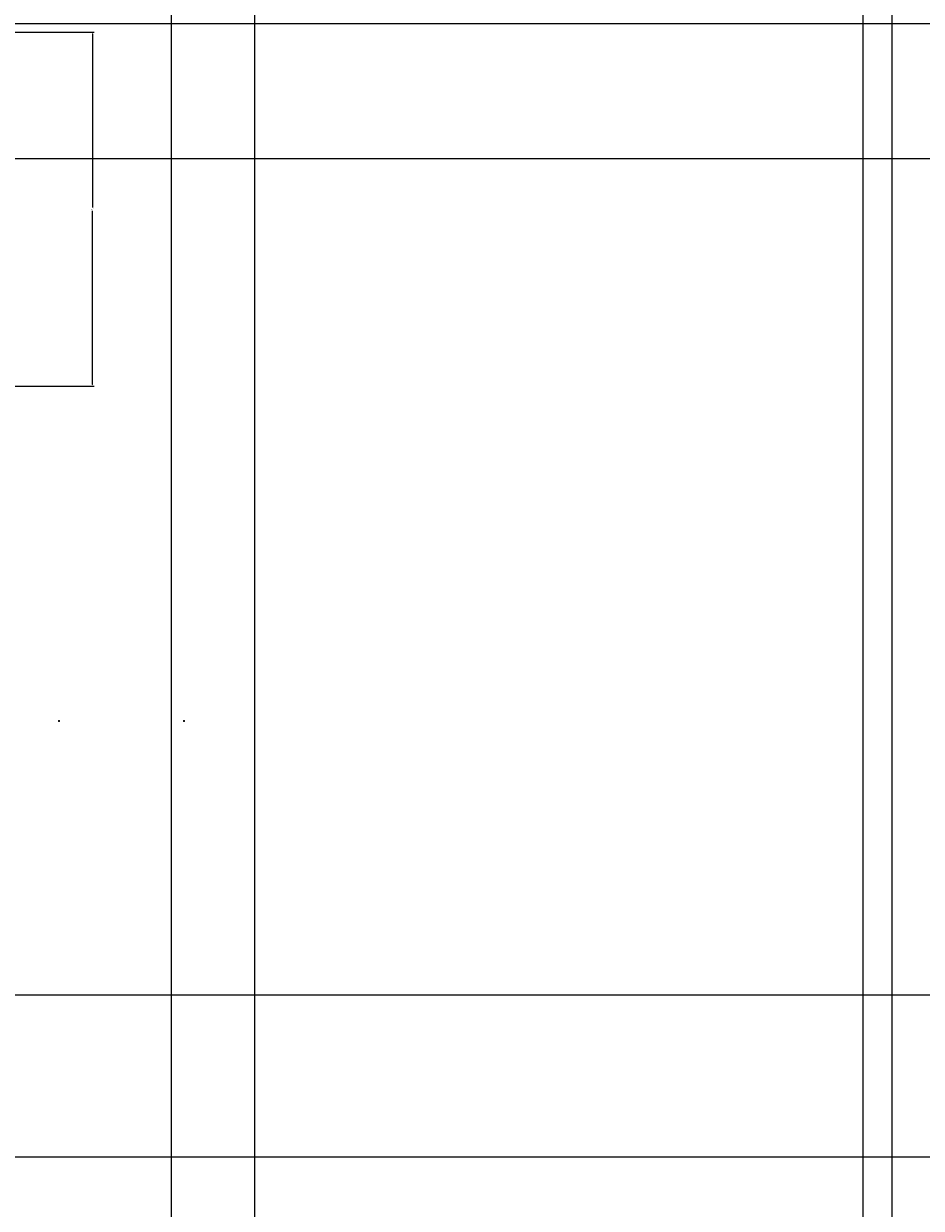
# Model space of a CAD drawing. Units: inches. Extents: x 1201 to 1754, y 247 to 775.
# Tile 5 of 10: x 1382 to 1475, y 435 to 557. Entities that reach past the tile are written whole.
import ezdxf

# ---------------------------------------------------------------- set-up
doc = ezdxf.new("R2010")
doc.units = ezdxf.units.IN
doc.layers.add('A-ANNO-DIMS', color=2, linetype='Continuous', lineweight=18)
doc.styles.get("Standard").update_dxf_attribs({"font": 'arial.ttf'})
doc.dimstyles.get("Standard").update_dxf_attribs({"dimtxt": 0.18, "dimasz": 0.18, "dimexe": 0.18, "dimexo": 0.0625, "dimgap": 0.09, "dimtad": 0, "dimtih": 1, "dimtoh": 1, "dimdec": 4, "dimzin": 0, "dimdsep": 46, "dimtxsty": 'Standard', "dimcen": 0.09, "dimadec": 0, "dimazin": 0, "dimtfac": 1, "dimtdec": 4, "dimtofl": 0, "dimtmove": 0, "dimatfit": 3, "dimfxl": 1, "dimtolj": 1, "dimtzin": 0, "dimarcsym": 0})

# ---------------------------------------------------------------- blocks, each defined once
blk = doc.blocks.new('*D32')
at = {"layer": 'A-ANNO-DIMS', "color": 0, "lineweight": -2, "transparency": 16777216}
for p, q in [((1379.77, 556.57), (1388.89, 556.57)), ((1388.71, 556.39), (1388.71, 538.42)), ((1388.71, 520.08), (1388.71, 538.05)), ((1379.77, 519.9), (1388.89, 519.9))]:
    blk.add_line(p, q, dxfattribs=at)
at = {"layer": 'A-ANNO-DIMS', "color": 0, "transparency": 16777216}
for points in [[(1388.68, 556.39), (1388.74, 556.39), (1388.71, 556.57)], [(1388.68, 520.08), (1388.74, 520.08), (1388.71, 519.9)]]:
    blk.add_solid(points, dxfattribs=at)
at = {"layer": 'Defpoints', "color": 0, "transparency": 16777216}
for p in [(1379.71, 556.57), (1388.71, 556.57), (1379.71, 519.9)]:
    blk.add_point(p, dxfattribs=at)
at = {"layer": 'A-ANNO-DIMS', "color": 0, "transparency": 16777216, "insert": (1388.71, 538.24), "char_height": 0.18, "attachment_point": 5}
blk.add_mtext('\\A1;37', dxfattribs=at)
blk = doc.blocks.new('*D58')
at = {"layer": 'A-ANNO-DIMS', "color": 0, "lineweight": -2, "transparency": 16777216}
for p, q in [((1405.52, 418), (1405.52, 775.14)), ((1405.7, 774.96), (1436.8, 774.96)), ((1468.34, 774.96), (1437.24, 774.96)), ((1468.52, 418), (1468.52, 775.14))]:
    blk.add_line(p, q, dxfattribs=at)
at = {"layer": 'A-ANNO-DIMS', "color": 0, "transparency": 16777216}
for points in [[(1405.7, 774.99), (1405.7, 774.93), (1405.52, 774.96)], [(1468.34, 774.99), (1468.34, 774.93), (1468.52, 774.96)]]:
    blk.add_solid(points, dxfattribs=at)
at = {"layer": 'Defpoints', "color": 0, "transparency": 16777216}
for p in [(1468.52, 774.96), (1405.52, 417.94), (1468.52, 417.94)]:
    blk.add_point(p, dxfattribs=at)
at = {"layer": 'A-ANNO-DIMS', "color": 0, "transparency": 16777216, "insert": (1437.02, 774.96), "char_height": 0.18, "attachment_point": 5}
blk.add_mtext('\\A1;63', dxfattribs=at)
blk = doc.blocks.new('*D59')
at = {"layer": 'A-ANNO-DIMS', "color": 0, "lineweight": -2, "transparency": 16777216}
for p, q in [((1255.52, 418), (1255.52, 775.14)), ((1255.7, 774.96), (1330.24, 774.96)), ((1405.34, 774.96), (1330.8, 774.96)), ((1405.52, 418), (1405.52, 775.14))]:
    blk.add_line(p, q, dxfattribs=at)
at = {"layer": 'A-ANNO-DIMS', "color": 0, "transparency": 16777216}
for points in [[(1255.7, 774.99), (1255.7, 774.93), (1255.52, 774.96)], [(1405.34, 774.99), (1405.34, 774.93), (1405.52, 774.96)]]:
    blk.add_solid(points, dxfattribs=at)
at = {"layer": 'Defpoints', "color": 0, "transparency": 16777216}
for p in [(1405.52, 774.96), (1255.52, 417.94), (1405.52, 417.94)]:
    blk.add_point(p, dxfattribs=at)
at = {"layer": 'A-ANNO-DIMS', "color": 0, "transparency": 16777216, "insert": (1330.52, 774.96), "char_height": 0.18, "attachment_point": 5}
blk.add_mtext('\\A1;150', dxfattribs=at)
blk = doc.blocks.new('*D75')
at = {"layer": 'A-ANNO-DIMS', "color": 0, "lineweight": -2, "transparency": 16777216}
for p, q in [((1717.46, 557.44), (1222.33, 557.44)), ((1222.51, 557.26), (1222.51, 550.62)), ((1222.51, 543.62), (1222.51, 550.26)), ((1717.46, 543.44), (1222.33, 543.44))]:
    blk.add_line(p, q, dxfattribs=at)
at = {"layer": 'A-ANNO-DIMS', "color": 0, "transparency": 16777216}
for points in [[(1222.48, 557.26), (1222.54, 557.26), (1222.51, 557.44)], [(1222.48, 543.62), (1222.54, 543.62), (1222.51, 543.44)]]:
    blk.add_solid(points, dxfattribs=at)
at = {"layer": 'Defpoints', "color": 0, "transparency": 16777216}
for p in [(1222.51, 557.44), (1717.52, 557.44), (1717.52, 543.44)]:
    blk.add_point(p, dxfattribs=at)
at = {"layer": 'A-ANNO-DIMS', "color": 0, "transparency": 16777216, "insert": (1222.51, 550.44), "char_height": 0.18, "attachment_point": 5}
blk.add_mtext('\\A1;14.005', dxfattribs=at)
blk = doc.blocks.new('*D83')
at = {"layer": 'A-ANNO-DIMS', "color": 0, "lineweight": -2, "transparency": 16777216}
for p, q in [((1471.46, 561.97), (1222.33, 561.97)), ((1222.51, 561.79), (1222.51, 559.89)), ((1222.51, 557.62), (1222.51, 559.52)), ((1471.46, 557.44), (1222.33, 557.44))]:
    blk.add_line(p, q, dxfattribs=at)
at = {"layer": 'A-ANNO-DIMS', "color": 0, "transparency": 16777216}
for points in [[(1222.48, 561.79), (1222.54, 561.79), (1222.51, 561.97)], [(1222.48, 557.62), (1222.54, 557.62), (1222.51, 557.44)]]:
    blk.add_solid(points, dxfattribs=at)
at = {"layer": 'Defpoints', "color": 0, "transparency": 16777216}
for p in [(1222.51, 561.97), (1471.52, 561.97), (1471.52, 557.44)]:
    blk.add_point(p, dxfattribs=at)
at = {"layer": 'A-ANNO-DIMS', "color": 0, "transparency": 16777216, "insert": (1222.51, 559.71), "char_height": 0.18, "attachment_point": 5}
blk.add_mtext('\\A1;4.528', dxfattribs=at)
blk = doc.blocks.new('*D89')
at = {"layer": 'A-ANNO-DIMS', "color": 0, "lineweight": -2, "transparency": 16777216}
for p, q in [((1396.89, 281.58), (1396.89, 775.14)), ((1397.07, 774.96), (1433.81, 774.96)), ((1471.34, 774.96), (1434.6, 774.96)), ((1471.52, 280), (1471.52, 775.14))]:
    blk.add_line(p, q, dxfattribs=at)
at = {"layer": 'A-ANNO-DIMS', "color": 0, "transparency": 16777216}
for points in [[(1397.07, 774.99), (1397.07, 774.93), (1396.89, 774.96)], [(1471.34, 774.99), (1471.34, 774.93), (1471.52, 774.96)]]:
    blk.add_solid(points, dxfattribs=at)
at = {"layer": 'Defpoints', "color": 0, "transparency": 16777216}
for p in [(1471.52, 774.96), (1396.89, 281.52), (1471.52, 279.94)]:
    blk.add_point(p, dxfattribs=at)
at = {"layer": 'A-ANNO-DIMS', "color": 0, "transparency": 16777216, "insert": (1434.21, 774.96), "char_height": 0.18, "attachment_point": 5}
blk.add_mtext('\\A1;74.63', dxfattribs=at)
blk = doc.blocks.new('*D95')
at = {"layer": 'A-ANNO-DIMS', "color": 0, "lineweight": -2, "transparency": 16777216}
for p, q in [((1366.15, 449.58), (1222.33, 449.58)), ((1222.51, 449.4), (1222.51, 433.94)), ((1222.51, 418.12), (1222.51, 433.58)), ((1405.46, 417.94), (1222.33, 417.94))]:
    blk.add_line(p, q, dxfattribs=at)
at = {"layer": 'A-ANNO-DIMS', "color": 0, "transparency": 16777216}
for points in [[(1222.48, 449.4), (1222.54, 449.4), (1222.51, 449.58)], [(1222.48, 418.12), (1222.54, 418.12), (1222.51, 417.94)]]:
    blk.add_solid(points, dxfattribs=at)
at = {"layer": 'Defpoints', "color": 0, "transparency": 16777216}
for p in [(1366.21, 449.58), (1222.51, 417.94), (1405.52, 417.94)]:
    blk.add_point(p, dxfattribs=at)
at = {"layer": 'A-ANNO-DIMS', "color": 0, "transparency": 16777216, "insert": (1222.51, 433.76), "char_height": 0.18, "attachment_point": 5}
blk.add_mtext('\\A1;31.64', dxfattribs=at)
blk = doc.blocks.new('*D96')
at = {"layer": 'A-ANNO-DIMS', "color": 0, "lineweight": -2, "transparency": 16777216}
for p, q in [((1714.98, 456.83), (1222.33, 456.83)), ((1222.51, 456.65), (1222.51, 448.61)), ((1222.51, 440.21), (1222.51, 448.25)), ((1717.46, 440.03), (1222.33, 440.03))]:
    blk.add_line(p, q, dxfattribs=at)
at = {"layer": 'A-ANNO-DIMS', "color": 0, "transparency": 16777216}
for points in [[(1222.48, 456.65), (1222.54, 456.65), (1222.51, 456.83)], [(1222.48, 440.21), (1222.54, 440.21), (1222.51, 440.03)]]:
    blk.add_solid(points, dxfattribs=at)
at = {"layer": 'Defpoints', "color": 0, "transparency": 16777216}
for p in [(1222.51, 456.83), (1715.05, 456.83), (1717.52, 440.03)]:
    blk.add_point(p, dxfattribs=at)
at = {"layer": 'A-ANNO-DIMS', "color": 0, "transparency": 16777216, "insert": (1222.51, 448.43), "char_height": 0.18, "attachment_point": 5}
blk.add_mtext('\\A1;16.793', dxfattribs=at)
blk = doc.blocks.new('*D100')
at = {"layer": 'A-ANNO-DIMS', "color": 0, "lineweight": -2, "transparency": 16777216}
for p, q in [((1204.3, 485.23), (1276.84, 485.23)), ((1398.12, 485.23), (1398.3, 485.23)), ((1398.21, 485.14), (1398.21, 485.32))]:
    blk.add_line(p, q, dxfattribs=at)
at = {"layer": 'A-ANNO-DIMS', "color": 0, "transparency": 16777216}
blk.add_solid([(1276.84, 485.26), (1276.84, 485.2), (1277.02, 485.23)], dxfattribs=at)
at = {"layer": 'Defpoints', "color": 0, "transparency": 16777216}
for p in [(1277.02, 485.23), (1398.21, 485.23)]:
    blk.add_point(p, dxfattribs=at)
at = {"layer": 'A-ANNO-DIMS', "color": 0, "transparency": 16777216, "insert": (1203.82, 485.23), "char_height": 0.18, "attachment_point": 5}
blk.add_mtext('\\A1;R121.2', dxfattribs=at)
blk = doc.blocks.new('*D101')
at = {"layer": 'A-ANNO-DIMS', "color": 0, "lineweight": -2, "transparency": 16777216}
for p, q in [((1202.47, 485.23), (1270.84, 485.23)), ((1385.18, 485.23), (1385.36, 485.23)), ((1385.27, 485.14), (1385.27, 485.32))]:
    blk.add_line(p, q, dxfattribs=at)
at = {"layer": 'A-ANNO-DIMS', "color": 0, "transparency": 16777216}
blk.add_solid([(1270.84, 485.26), (1270.84, 485.2), (1271.02, 485.23)], dxfattribs=at)
at = {"layer": 'Defpoints', "color": 0, "transparency": 16777216}
for p in [(1271.02, 485.23), (1385.27, 485.23)]:
    blk.add_point(p, dxfattribs=at)
at = {"layer": 'A-ANNO-DIMS', "color": 0, "transparency": 16777216, "insert": (1201.92, 485.23), "char_height": 0.18, "attachment_point": 5}
blk.add_mtext('\\A1;R114.25', dxfattribs=at)

msp = doc.modelspace()

# ---------------------------------------------------------------- dimensions: what is measured, and where the dimension line sits
at = {"layer": 'A-ANNO-DIMS'}
for base, p1, p2, override, picture, middle in [((1405.5208, 774.9565), (1255.5208, 417.9415), (1405.5208, 417.9415), {"dimdec": 0, "dimlfac": 1, "dimrnd": 0, "dimzin": 0, "dimdsep": 46, "dimlunit": 2}, '*D59', (1330.5208, 774.9565)), ((1471.5208, 774.9565), (1396.8927, 281.5161), (1471.5208, 279.9415), {"dimdec": 2, "dimlfac": 1, "dimrnd": 0, "dimzin": 0, "dimdsep": 46, "dimlunit": 2}, '*D89', (1434.2067, 774.9565)), ((1468.5208, 774.9565), (1405.5208, 417.9415), (1468.5208, 417.9415), {"dimdec": 0, "dimlfac": 1, "dimrnd": 0, "dimzin": 0, "dimdsep": 46, "dimlunit": 2}, '*D58', (1437.0208, 774.9565))]:
    dim = msp.add_linear_dim(base=base, p1=p1, p2=p2, dimstyle='Standard', override=override, dxfattribs=at)
    dim.commit()
    dim.dimension.update_dxf_attribs({"geometry": picture, "text_midpoint": middle})
for base, p1, p2, override, picture, middle in [((1222.5058, 561.9692), (1471.5208, 557.4415), (1471.5208, 561.9692), {"dimdec": 3, "dimlfac": 1, "dimrnd": 0, "dimzin": 0, "dimdsep": 46, "dimlunit": 2}, '*D83', (1222.5058, 559.7053)), ((1222.5058, 557.4415), (1717.5208, 543.4363), (1717.5208, 557.4415), {"dimdec": 3, "dimlfac": 1, "dimrnd": 0, "dimzin": 0, "dimdsep": 46, "dimlunit": 2}, '*D75', (1222.5058, 550.4389)), ((1388.7057, 556.5701), (1379.7057, 519.9035), (1379.7057, 556.5701), {"dimdec": 0, "dimlfac": 1, "dimrnd": 0, "dimzin": 0, "dimdsep": 46, "dimlunit": 2}, '*D32', (1388.7057, 538.2368)), ((1222.5058, 456.8273), (1717.5208, 440.0342), (1715.0469, 456.8273), {"dimdec": 3, "dimlfac": 1, "dimrnd": 0, "dimzin": 0, "dimdsep": 46, "dimlunit": 2}, '*D96', (1222.5058, 448.4308)), ((1222.5058, 417.9415), (1366.2113, 449.5839), (1405.5208, 417.9415), {"dimdec": 2, "dimlfac": 1, "dimrnd": 0, "dimzin": 0, "dimdsep": 46, "dimlunit": 2}, '*D95', (1222.5058, 433.7627))]:
    dim = msp.add_linear_dim(base=base, p1=p1, p2=p2, angle=90, dimstyle='Standard', override=override, dxfattribs=at)
    dim.commit()
    dim.dimension.update_dxf_attribs({"geometry": picture, "text_midpoint": middle})
for center, mpoint, override, picture, middle in [((1385.2665, 485.2267), (1271.0165, 485.227), {"dimdec": 2, "dimlfac": 1, "dimrnd": 0, "dimzin": 0, "dimdsep": 46, "dimlunit": 2}, '*D101', (1202.4665, 485.2272)), ((1398.2133, 485.2267), (1277.0165, 485.227), {"dimdec": 1, "dimlfac": 1, "dimrnd": 0, "dimzin": 0, "dimdsep": 46, "dimlunit": 2}, '*D100', (1204.2984, 485.2272))]:
    dim = msp.add_radius_dim(center=center, mpoint=mpoint, dimstyle='Standard', override=override, dxfattribs=at)
    dim.commit()
    dim.dimension.update_dxf_attribs({"geometry": picture, "text_midpoint": middle, "dimtype": 164})

doc.saveas('drawing.dxf')
